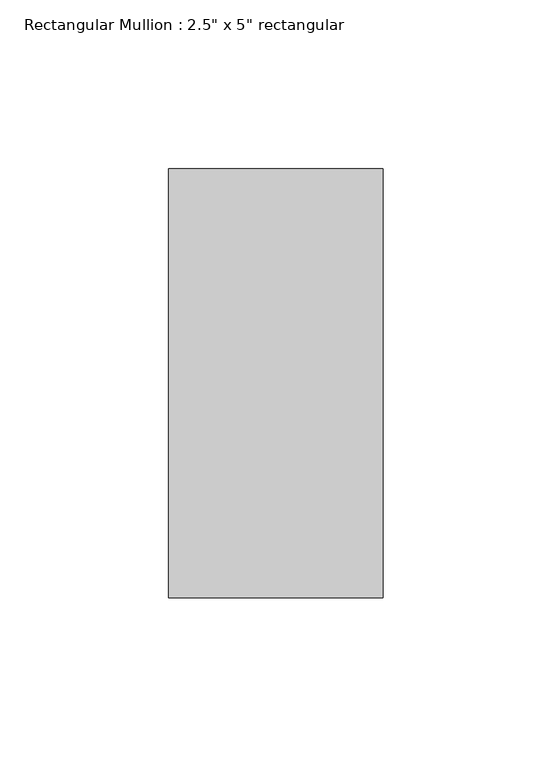
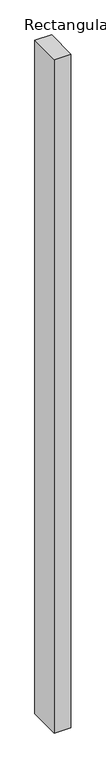
"""IFC4 building model written with IfcOpenShell, lengths in millimetres: member geometry."""

from ifc_helpers import new_model, si_unit, frame, origin, place, context, project, spatial, polyline, outline, extrude, source, transform, mapped, element, save


def member_1bc55d26(model_context):
    return source(origin(), model_context, "Body", "SweptSolid", [
        extrude(outline(polyline([(31.75, 63.5), (31.75, -63.5), (-31.75, -63.5), (-31.75, 63.5), (31.75, 63.5)])), frame((0.0, 0.0, -2704.8948327), z_axis=(0.0, 0.0, 1.0), x_axis=(1.0, 0.0, 0.0)), (0.0, 0.0, 1.0), 2704.8948327),
    ])


if __name__ == "__main__":
    model = new_model("IFC4")
    model_context = context("Model", 3, world=origin())
    ifc_project = project(units=[si_unit("LENGTHUNIT", "METRE", prefix="MILLI")], contexts=[model_context])
    site = spatial("IfcSite", under=ifc_project)
    building = spatial("IfcBuilding", under=site)
    placement = place(None, origin())
    member_shape = member_1bc55d26(model_context)
    element("IfcMember", 1, ObjectType="Rectangular Mullion : 2.5\" x 5\" rectangular", at=placement, inside=building, context=model_context, shape_type="MappedRepresentation", body=[
        mapped(member_shape, transform((0.0, 0.0, 0.0), x_axis=(1.0, 0.0, 0.0), y_axis=(0.0, 1.0, 0.0), z_axis=(0.0, 0.0, 1.0))),
    ])
    save(model, "model.ifc")

# Revit data of these elements
# Type "Rectangular Mullion : 2.5\" x 5\" rectangular"
#   built-in parameter 1007304 = 0.416667 (stored number, unit not read)
#   built-in parameter 1007301 = 0.104167 (stored number, unit not read)
#   built-in parameter 1007300 = 0.104167 (stored number, unit not read)
# Element 1 (IfcMember, "Rectangular Mullion : 2.5\" x 5\" rectangular")
#   Materials on its faces: "Damp-proofing"
# Materials
#   "Damp-proofing": class "Generic", colour RGB 127 127 127, transparency 0, Description = "Damp-proofing", Cost = 0
